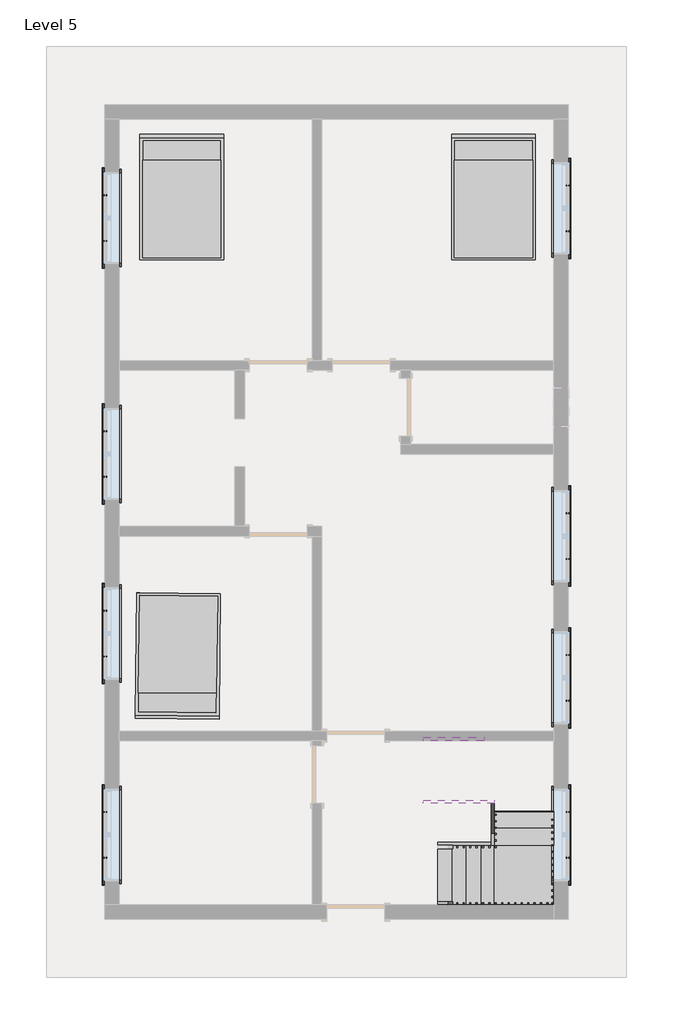
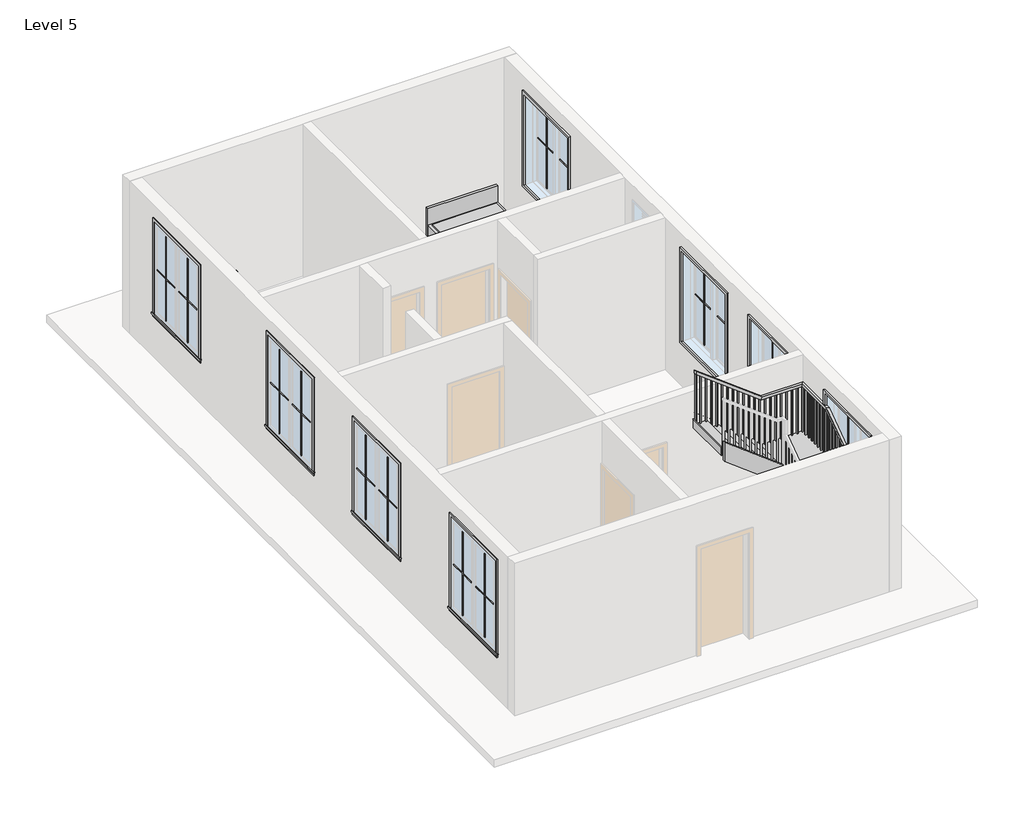
# One storey, part 2 of 2: 32 proxies, 5 members, 3 furniture elements, 1 railing, 1 stair flight.
"""IFC4 building model written with IfcOpenShell, lengths in millimetres."""

from ifc_helpers import new_model, si_unit, frame, origin, place, context, project, spatial, polyline, outline, extrude, faceted_brep, transform, mapped, element, save
from components import muntin_pattern_2x2_muntin_pattern_2x2_bff912c5, muntin_pattern_2x2_muntin_pattern_2x2_c2194282, trim_window_exterior_flat_with_sill_e04b3088, trim_window_interior_flat_picture_frame_2a7685fe, bed_17739_bed_17739_15c61121, stair_flight_f19c2654

model = new_model("IFC4")

# Units and contexts
model_context = context("Model", 3, world=origin())
ifc_project = project(units=[si_unit("LENGTHUNIT", "METRE", prefix="MILLI")], contexts=[model_context])

# Site, building, storey
site = spatial("IfcSite", under=ifc_project)
building = spatial("IfcBuilding", under=site)
storey = spatial("IfcBuildingStorey", under=building, Name="Level 5", Elevation=9601.2)

# Proxies
placement = place(None, origin())
muntin_pattern_2x2_muntin_pattern_2x2_shape = muntin_pattern_2x2_muntin_pattern_2x2_bff912c5(model_context)
element("IfcBuildingElementProxy", 1, Name="Muntin Pattern_2x2 : Muntin Pattern_2x2", ObjectType="Muntin Pattern_2x2 : Muntin Pattern_2x2", at=placement, inside=storey, context=model_context, shape_type="MappedRepresentation", body=[
    mapped(muntin_pattern_2x2_muntin_pattern_2x2_shape, transform((-4903.510885, -5396.5975571, 10585.45), x_axis=(0.0, 1.0, 0.0), y_axis=(-1.0, 0.0, 0.0), z_axis=(0.0, 0.0, 1.0))),
])
element("IfcBuildingElementProxy", 2, Name="Muntin Pattern_2x2 : Muntin Pattern_2x2", ObjectType="Muntin Pattern_2x2 : Muntin Pattern_2x2", at=placement, inside=storey, context=model_context, shape_type="MappedRepresentation", body=[
    mapped(muntin_pattern_2x2_muntin_pattern_2x2_shape, transform((2392.639115, -4675.8725571, 10585.45), x_axis=(0.0, -1.0, 0.0), y_axis=(1.0, 0.0, 0.0), z_axis=(0.0, 0.0, 1.0))),
])
element("IfcBuildingElementProxy", 3, Name="Muntin Pattern_2x2 : Muntin Pattern_2x2", ObjectType="Muntin Pattern_2x2 : Muntin Pattern_2x2", at=placement, inside=storey, context=model_context, shape_type="MappedRepresentation", body=[
    mapped(muntin_pattern_2x2_muntin_pattern_2x2_shape, transform((2392.639115, -2199.3725571, 10585.45), x_axis=(0.0, -1.0, 0.0), y_axis=(1.0, 0.0, 0.0), z_axis=(0.0, 0.0, 1.0))),
])
element("IfcBuildingElementProxy", 4, Name="Muntin Pattern_2x2 : Muntin Pattern_2x2", ObjectType="Muntin Pattern_2x2 : Muntin Pattern_2x2", at=placement, inside=storey, context=model_context, shape_type="MappedRepresentation", body=[
    mapped(muntin_pattern_2x2_muntin_pattern_2x2_shape, transform((2392.639115, 35.8274429, 10585.45), x_axis=(0.0, -1.0, 0.0), y_axis=(1.0, 0.0, 0.0), z_axis=(0.0, 0.0, 1.0))),
])
element("IfcBuildingElementProxy", 5, Name="Muntin Pattern_2x2 : Muntin Pattern_2x2", ObjectType="Muntin Pattern_2x2 : Muntin Pattern_2x2", at=placement, inside=storey, context=model_context, shape_type="MappedRepresentation", body=[
    mapped(muntin_pattern_2x2_muntin_pattern_2x2_shape, transform((-4903.510885, -2221.5975571, 10585.45), x_axis=(0.0, 1.0, 0.0), y_axis=(-1.0, 0.0, 0.0), z_axis=(0.0, 0.0, 1.0))),
])
element("IfcBuildingElementProxy", 6, Name="Muntin Pattern_2x2 : Muntin Pattern_2x2", ObjectType="Muntin Pattern_2x2 : Muntin Pattern_2x2", at=placement, inside=storey, context=model_context, shape_type="MappedRepresentation", body=[
    mapped(muntin_pattern_2x2_muntin_pattern_2x2_shape, transform((-4903.510885, 610.5024429, 10585.45), x_axis=(0.0, 1.0, 0.0), y_axis=(-1.0, 0.0, 0.0), z_axis=(0.0, 0.0, 1.0))),
])
element("IfcBuildingElementProxy", 7, Name="Muntin Pattern_2x2 : Muntin Pattern_2x2", ObjectType="Muntin Pattern_2x2 : Muntin Pattern_2x2", at=placement, inside=storey, context=model_context, shape_type="MappedRepresentation", body=[
    mapped(muntin_pattern_2x2_muntin_pattern_2x2_shape, transform((-4903.510885, 4331.6024429, 10585.45), x_axis=(0.0, 1.0, 0.0), y_axis=(-1.0, 0.0, 0.0), z_axis=(0.0, 0.0, 1.0))),
])
element("IfcBuildingElementProxy", 8, Name="Muntin Pattern_2x2 : Muntin Pattern_2x2", ObjectType="Muntin Pattern_2x2 : Muntin Pattern_2x2", at=placement, inside=storey, context=model_context, shape_type="MappedRepresentation", body=[
    mapped(muntin_pattern_2x2_muntin_pattern_2x2_shape, transform((2392.639115, 5204.7274429, 10585.45), x_axis=(0.0, -1.0, 0.0), y_axis=(1.0, 0.0, 0.0), z_axis=(0.0, 0.0, 1.0))),
])
muntin_pattern_2x2_muntin_pattern_2x2_2_shape = muntin_pattern_2x2_muntin_pattern_2x2_c2194282(model_context)
element("IfcBuildingElementProxy", 9, Name="Muntin Pattern_2x2 : Muntin Pattern_2x2", ObjectType="Muntin Pattern_2x2 : Muntin Pattern_2x2", at=placement, inside=storey, context=model_context, shape_type="MappedRepresentation", body=[
    mapped(muntin_pattern_2x2_muntin_pattern_2x2_2_shape, transform((-4903.510885, -4675.8725571, 10585.45), x_axis=(0.0, -1.0, 0.0), y_axis=(1.0, 0.0, 0.0), z_axis=(0.0, 0.0, 1.0))),
])
element("IfcBuildingElementProxy", 10, Name="Muntin Pattern_2x2 : Muntin Pattern_2x2", ObjectType="Muntin Pattern_2x2 : Muntin Pattern_2x2", at=placement, inside=storey, context=model_context, shape_type="MappedRepresentation", body=[
    mapped(muntin_pattern_2x2_muntin_pattern_2x2_2_shape, transform((2392.639115, -5396.5975571, 10585.45), x_axis=(0.0, 1.0, 0.0), y_axis=(-1.0, 0.0, 0.0), z_axis=(0.0, 0.0, 1.0))),
])
element("IfcBuildingElementProxy", 11, Name="Muntin Pattern_2x2 : Muntin Pattern_2x2", ObjectType="Muntin Pattern_2x2 : Muntin Pattern_2x2", at=placement, inside=storey, context=model_context, shape_type="MappedRepresentation", body=[
    mapped(muntin_pattern_2x2_muntin_pattern_2x2_2_shape, transform((2392.639115, -2920.0975571, 10585.45), x_axis=(0.0, 1.0, 0.0), y_axis=(-1.0, 0.0, 0.0), z_axis=(0.0, 0.0, 1.0))),
])
element("IfcBuildingElementProxy", 12, Name="Muntin Pattern_2x2 : Muntin Pattern_2x2", ObjectType="Muntin Pattern_2x2 : Muntin Pattern_2x2", at=placement, inside=storey, context=model_context, shape_type="MappedRepresentation", body=[
    mapped(muntin_pattern_2x2_muntin_pattern_2x2_2_shape, transform((2392.639115, -684.8975571, 10585.45), x_axis=(0.0, 1.0, 0.0), y_axis=(-1.0, 0.0, 0.0), z_axis=(0.0, 0.0, 1.0))),
])
element("IfcBuildingElementProxy", 13, Name="Muntin Pattern_2x2 : Muntin Pattern_2x2", ObjectType="Muntin Pattern_2x2 : Muntin Pattern_2x2", at=placement, inside=storey, context=model_context, shape_type="MappedRepresentation", body=[
    mapped(muntin_pattern_2x2_muntin_pattern_2x2_2_shape, transform((-4903.510885, -1500.8725571, 10585.45), x_axis=(0.0, -1.0, 0.0), y_axis=(1.0, 0.0, 0.0), z_axis=(0.0, 0.0, 1.0))),
])
element("IfcBuildingElementProxy", 14, Name="Muntin Pattern_2x2 : Muntin Pattern_2x2", ObjectType="Muntin Pattern_2x2 : Muntin Pattern_2x2", at=placement, inside=storey, context=model_context, shape_type="MappedRepresentation", body=[
    mapped(muntin_pattern_2x2_muntin_pattern_2x2_2_shape, transform((-4903.510885, 1331.2274429, 10585.45), x_axis=(0.0, -1.0, 0.0), y_axis=(1.0, 0.0, 0.0), z_axis=(0.0, 0.0, 1.0))),
])
element("IfcBuildingElementProxy", 15, Name="Muntin Pattern_2x2 : Muntin Pattern_2x2", ObjectType="Muntin Pattern_2x2 : Muntin Pattern_2x2", at=placement, inside=storey, context=model_context, shape_type="MappedRepresentation", body=[
    mapped(muntin_pattern_2x2_muntin_pattern_2x2_2_shape, transform((-4903.510885, 5052.3274429, 10585.45), x_axis=(0.0, -1.0, 0.0), y_axis=(1.0, 0.0, 0.0), z_axis=(0.0, 0.0, 1.0))),
])
element("IfcBuildingElementProxy", 16, Name="Muntin Pattern_2x2 : Muntin Pattern_2x2", ObjectType="Muntin Pattern_2x2 : Muntin Pattern_2x2", at=placement, inside=storey, context=model_context, shape_type="MappedRepresentation", body=[
    mapped(muntin_pattern_2x2_muntin_pattern_2x2_2_shape, transform((2392.639115, 4484.0024429, 10585.45), x_axis=(0.0, 1.0, 0.0), y_axis=(-1.0, 0.0, 0.0), z_axis=(0.0, 0.0, 1.0))),
])
trim_window_exterior_flat_with_sill_shape = trim_window_exterior_flat_with_sill_e04b3088(model_context)
element("IfcBuildingElementProxy", 17, Name="Trim-Window-Exterior-Flat : with Sill", ObjectType="Trim-Window-Exterior-Flat : with Sill", at=placement, inside=storey, context=model_context, shape_type="MappedRepresentation", body=[
    mapped(trim_window_exterior_flat_with_sill_shape, transform((-4913.035885, -5036.2350571, 12344.4), x_axis=(0.0, -1.0, 0.0), y_axis=(0.0, 0.0, 1.0), z_axis=(-1.0, 0.0, 0.0))),
])
element("IfcBuildingElementProxy", 18, Name="Trim-Window-Exterior-Flat : with Sill", ObjectType="Trim-Window-Exterior-Flat : with Sill", at=placement, inside=storey, context=model_context, shape_type="MappedRepresentation", body=[
    mapped(trim_window_exterior_flat_with_sill_shape, transform((2402.164115, -5036.2350571, 12344.4), x_axis=(0.0, 1.0, 0.0), y_axis=(0.0, 0.0, 1.0), z_axis=(1.0, 0.0, 0.0))),
])
element("IfcBuildingElementProxy", 19, Name="Trim-Window-Exterior-Flat : with Sill", ObjectType="Trim-Window-Exterior-Flat : with Sill", at=placement, inside=storey, context=model_context, shape_type="MappedRepresentation", body=[
    mapped(trim_window_exterior_flat_with_sill_shape, transform((2402.164115, -2559.7350571, 12344.4), x_axis=(0.0, 1.0, 0.0), y_axis=(0.0, 0.0, 1.0), z_axis=(1.0, 0.0, 0.0))),
])
element("IfcBuildingElementProxy", 20, Name="Trim-Window-Exterior-Flat : with Sill", ObjectType="Trim-Window-Exterior-Flat : with Sill", at=placement, inside=storey, context=model_context, shape_type="MappedRepresentation", body=[
    mapped(trim_window_exterior_flat_with_sill_shape, transform((2402.164115, -324.5350571, 12344.4), x_axis=(0.0, 1.0, 0.0), y_axis=(0.0, 0.0, 1.0), z_axis=(1.0, 0.0, 0.0))),
])
element("IfcBuildingElementProxy", 21, Name="Trim-Window-Exterior-Flat : with Sill", ObjectType="Trim-Window-Exterior-Flat : with Sill", at=placement, inside=storey, context=model_context, shape_type="MappedRepresentation", body=[
    mapped(trim_window_exterior_flat_with_sill_shape, transform((-4913.035885, -1861.2350571, 12344.4), x_axis=(0.0, -1.0, 0.0), y_axis=(0.0, 0.0, 1.0), z_axis=(-1.0, 0.0, 0.0))),
])
element("IfcBuildingElementProxy", 22, Name="Trim-Window-Exterior-Flat : with Sill", ObjectType="Trim-Window-Exterior-Flat : with Sill", at=placement, inside=storey, context=model_context, shape_type="MappedRepresentation", body=[
    mapped(trim_window_exterior_flat_with_sill_shape, transform((-4913.035885, 970.8649429, 12344.4), x_axis=(0.0, -1.0, 0.0), y_axis=(0.0, 0.0, 1.0), z_axis=(-1.0, 0.0, 0.0))),
])
element("IfcBuildingElementProxy", 23, Name="Trim-Window-Exterior-Flat : with Sill", ObjectType="Trim-Window-Exterior-Flat : with Sill", at=placement, inside=storey, context=model_context, shape_type="MappedRepresentation", body=[
    mapped(trim_window_exterior_flat_with_sill_shape, transform((-4913.035885, 4691.9649429, 12344.4), x_axis=(0.0, -1.0, 0.0), y_axis=(0.0, 0.0, 1.0), z_axis=(-1.0, 0.0, 0.0))),
])
element("IfcBuildingElementProxy", 24, Name="Trim-Window-Exterior-Flat : with Sill", ObjectType="Trim-Window-Exterior-Flat : with Sill", at=placement, inside=storey, context=model_context, shape_type="MappedRepresentation", body=[
    mapped(trim_window_exterior_flat_with_sill_shape, transform((2402.164115, 4844.3649429, 12344.4), x_axis=(0.0, 1.0, 0.0), y_axis=(0.0, 0.0, 1.0), z_axis=(1.0, 0.0, 0.0))),
])
trim_window_interior_flat_picture_frame_shape = trim_window_interior_flat_picture_frame_2a7685fe(model_context)
element("IfcBuildingElementProxy", 25, Name="Trim-Window-Interior-Flat : Picture Frame", ObjectType="Trim-Window-Interior-Flat : Picture Frame", at=placement, inside=storey, context=model_context, shape_type="MappedRepresentation", body=[
    mapped(trim_window_interior_flat_picture_frame_shape, transform((-4684.435885, -5036.2350571, 12344.4), x_axis=(0.0, 1.0, 0.0), y_axis=(0.0, 0.0, 1.0), z_axis=(1.0, 0.0, 0.0))),
])
element("IfcBuildingElementProxy", 26, Name="Trim-Window-Interior-Flat : Picture Frame", ObjectType="Trim-Window-Interior-Flat : Picture Frame", at=placement, inside=storey, context=model_context, shape_type="MappedRepresentation", body=[
    mapped(trim_window_interior_flat_picture_frame_shape, transform((2173.564115, -5036.2350571, 12344.4), x_axis=(0.0, -1.0, 0.0), y_axis=(0.0, 0.0, 1.0), z_axis=(-1.0, 0.0, 0.0))),
])
element("IfcBuildingElementProxy", 27, Name="Trim-Window-Interior-Flat : Picture Frame", ObjectType="Trim-Window-Interior-Flat : Picture Frame", at=placement, inside=storey, context=model_context, shape_type="MappedRepresentation", body=[
    mapped(trim_window_interior_flat_picture_frame_shape, transform((2173.564115, -2559.7350571, 12344.4), x_axis=(0.0, -1.0, 0.0), y_axis=(0.0, 0.0, 1.0), z_axis=(-1.0, 0.0, 0.0))),
])
element("IfcBuildingElementProxy", 28, Name="Trim-Window-Interior-Flat : Picture Frame", ObjectType="Trim-Window-Interior-Flat : Picture Frame", at=placement, inside=storey, context=model_context, shape_type="MappedRepresentation", body=[
    mapped(trim_window_interior_flat_picture_frame_shape, transform((2173.564115, -324.5350571, 12344.4), x_axis=(0.0, -1.0, 0.0), y_axis=(0.0, 0.0, 1.0), z_axis=(-1.0, 0.0, 0.0))),
])
element("IfcBuildingElementProxy", 29, Name="Trim-Window-Interior-Flat : Picture Frame", ObjectType="Trim-Window-Interior-Flat : Picture Frame", at=placement, inside=storey, context=model_context, shape_type="MappedRepresentation", body=[
    mapped(trim_window_interior_flat_picture_frame_shape, transform((-4684.435885, -1861.2350571, 12344.4), x_axis=(0.0, 1.0, 0.0), y_axis=(0.0, 0.0, 1.0), z_axis=(1.0, 0.0, 0.0))),
])
element("IfcBuildingElementProxy", 30, Name="Trim-Window-Interior-Flat : Picture Frame", ObjectType="Trim-Window-Interior-Flat : Picture Frame", at=placement, inside=storey, context=model_context, shape_type="MappedRepresentation", body=[
    mapped(trim_window_interior_flat_picture_frame_shape, transform((-4684.435885, 970.8649429, 12344.4), x_axis=(0.0, 1.0, 0.0), y_axis=(0.0, 0.0, 1.0), z_axis=(1.0, 0.0, 0.0))),
])
element("IfcBuildingElementProxy", 31, Name="Trim-Window-Interior-Flat : Picture Frame", ObjectType="Trim-Window-Interior-Flat : Picture Frame", at=placement, inside=storey, context=model_context, shape_type="MappedRepresentation", body=[
    mapped(trim_window_interior_flat_picture_frame_shape, transform((-4684.435885, 4691.9649429, 12344.4), x_axis=(0.0, 1.0, 0.0), y_axis=(0.0, 0.0, 1.0), z_axis=(1.0, 0.0, 0.0))),
])
element("IfcBuildingElementProxy", 32, Name="Trim-Window-Interior-Flat : Picture Frame", ObjectType="Trim-Window-Interior-Flat : Picture Frame", at=placement, inside=storey, context=model_context, shape_type="MappedRepresentation", body=[
    mapped(trim_window_interior_flat_picture_frame_shape, transform((2173.564115, 4844.3649429, 12344.4), x_axis=(0.0, -1.0, 0.0), y_axis=(0.0, 0.0, 1.0), z_axis=(-1.0, 0.0, 0.0))),
])

# Furniture
bed_17739_bed_17739_shape = bed_17739_bed_17739_15c61121(model_context)
element("IfcFurniture", 33, ObjectType="Bed_17739 : Bed_17739", at=placement, inside=storey, context=model_context, shape_type="MappedRepresentation", body=[
    mapped(bed_17739_bed_17739_shape, transform((-3693.835885, 4996.7649429, 9601.2), x_axis=(1.0, 0.0, 0.0), y_axis=(0.0, 1.0, 0.0), z_axis=(0.0, 0.0, 1.0))),
])
element("IfcFurniture", 34, ObjectType="Bed_17739 : Bed_17739", at=placement, inside=storey, context=model_context, shape_type="MappedRepresentation", body=[
    mapped(bed_17739_bed_17739_shape, transform((1221.064115, 4996.7649429, 9601.2), x_axis=(1.0, 0.0, 0.0), y_axis=(0.0, 1.0, 0.0), z_axis=(0.0, 0.0, 1.0))),
])
element("IfcFurniture", 35, ObjectType="Bed_17739 : Bed_17739", at=placement, inside=storey, context=model_context, shape_type="MappedRepresentation", body=[
    mapped(bed_17739_bed_17739_shape, transform((-3756.0321663, -2189.364606, 9601.2), x_axis=(-0.9999334593473937, 0.011535895177843815, 0.0), y_axis=(-0.011535895177843815, -0.9999334593473937, 0.0), z_axis=(0.0, 0.0, 1.0))),
])

# Members
element("IfcMember", 36, ObjectType="Stringer - 2\" Width", at=placement, inside=storey, context=model_context, shape_type="SweptSolid", body=[
    extrude(outline(polyline([(9823.8959685, 344.764115), (9601.2, 344.764115), (9601.2, 555.1685253), (10084.1196844, 1182.964115), (10468.6651993, 1182.964115), (9823.8959685, 344.764115)])), frame((0.0, -5201.3350571, 0.0), z_axis=(0.0, 1.0, 0.0), x_axis=(0.0, 0.0, 1.0)), (0.0, 0.0, 1.0), 50.8),
])
element("IfcMember", 37, ObjectType="Stringer - 2\" Width", at=placement, inside=storey, context=model_context, shape_type="SweptSolid", body=[
    extrude(outline(polyline([(-5201.3350571, 10296.352716), (-5201.3350571, 10670.9225362), (-4540.9350571, 11142.6368219), (-4540.9350571, 10768.0670017), (-5201.3350571, 10296.352716)])), frame((1182.964115, 0.0, 0.0), z_axis=(1.0, 0.0, 0.0), x_axis=(0.0, 1.0, 0.0)), (0.0, 0.0, 1.0), 50.8),
])
element("IfcMember", 38, ObjectType="Stringer - 2\" Width", at=placement, inside=storey, context=model_context, shape_type="SweptSolid", body=[
    extrude(outline(polyline([(10970.3786616, 1233.764115), (11353.5668, 1233.764115), (12205.0715619, 116.164115), (11821.8834236, 116.164115), (10970.3786616, 1233.764115)])), frame((0.0, -4540.9350571, 0.0), z_axis=(0.0, 1.0, 0.0), x_axis=(0.0, 0.0, 1.0)), (0.0, 0.0, 1.0), 50.8),
])
element("IfcMember", 39, ObjectType="Stringer - 2\" Width", at=placement, inside=storey, context=model_context, shape_type="SweptSolid", body=[
    extrude(outline(polyline([(9823.8959685, 344.764115), (9601.2, 344.764115), (9601.2, 555.1685253), (9999.6368219, 1073.1363938), (9999.6368219, 573.2272245), (9823.8959685, 344.764115)])), frame((0.0, -6191.9350571, 0.0), z_axis=(0.0, 1.0, 0.0), x_axis=(0.0, 0.0, 1.0)), (0.0, 0.0, 1.0), 50.8),
])
element("IfcMember", 40, ObjectType="Stringer - 2\" Width", at=placement, inside=storey, context=model_context, shape_type="SweptSolid", body=[
    extrude(outline(polyline([(11475.6384303, 1073.5451003), (12205.0715619, 116.164115), (11821.8834236, 116.164115), (11475.6384303, 570.6106687), (11475.6384303, 1073.5451003)])), frame((0.0, -3550.3350571, 0.0), z_axis=(0.0, 1.0, 0.0), x_axis=(0.0, 0.0, 1.0)), (0.0, 0.0, 1.0), 50.8),
])

# Railing
element("IfcRailing", 41, ObjectType="Handrail - Rectangular", at=placement, inside=storey, context=model_context, shape_type="SolidModel", body=[
    faceted_brep([(344.764115, -6090.3350571, 10684.9333333), (344.764115, -6090.3350571, 10621.0686436), (344.764115, -6141.1350571, 10621.0686436), (344.764115, -6141.1350571, 10684.9333333), (1373.464115, -6090.3350571, 11468.7047619), (1390.6115203, -6090.3350571, 11417.9047619), (1390.6115203, -6141.1350571, 11417.9047619), (1373.464115, -6141.1350571, 11468.7047619), (2122.764115, -6090.3350571, 11468.7047619), (2122.764115, -6090.3350571, 11417.9047619), (2173.564115, -6141.1350571, 11417.9047619), (2173.564115, -6141.1350571, 11468.7047619), (2122.764115, -5289.3883904, 11468.7047619), (2122.764115, -5273.1087657, 11417.9047619), (2173.564115, -5273.1087657, 11417.9047619), (2173.564115, -5289.3883904, 11468.7047619), (2122.764115, -4399.3108146, 12104.4744589), (2122.764115, -4383.0311899, 12053.6744589), (2173.564115, -4383.0311899, 12053.6744589), (2173.564115, -4399.3108146, 12104.4744589), (2122.764115, -3601.1350571, 12104.4744589), (2122.764115, -3601.1350571, 12053.6744589), (2173.564115, -3550.3350571, 12053.6744589), (2173.564115, -3550.3350571, 12104.4744589), (1371.6498293, -3601.1350571, 12104.4744589), (1354.5800477, -3601.1350571, 12053.6744589), (1354.5800477, -3550.3350571, 12053.6744589), (1371.6498293, -3550.3350571, 12104.4744589), (116.164115, -3601.1350571, 13055.6), (116.164115, -3550.3350571, 13055.6), (116.164115, -3550.3350571, 12991.8683472), (116.164115, -3601.1350571, 12991.8683472)], [[[0, 1, 2, 3]], [[1, 0, 4, 5]], [[2, 1, 5, 6]], [[3, 2, 6, 7]], [[0, 3, 7, 4]], [[5, 4, 8, 9]], [[6, 5, 9, 10]], [[7, 6, 10, 11]], [[4, 7, 11, 8]], [[9, 8, 12, 13]], [[10, 9, 13, 14]], [[11, 10, 14, 15]], [[8, 11, 15, 12]], [[13, 12, 16, 17]], [[14, 13, 17, 18]], [[15, 14, 18, 19]], [[12, 15, 19, 16]], [[17, 16, 20, 21]], [[18, 17, 21, 22]], [[19, 18, 22, 23]], [[16, 19, 23, 20]], [[21, 20, 24, 25]], [[22, 21, 25, 26]], [[23, 22, 26, 27]], [[20, 23, 27, 24]], [[28, 29, 30, 31]], [[25, 24, 28, 31]], [[26, 25, 31, 30]], [[27, 26, 30, 29]], [[24, 27, 29, 28]]]),
    extrude(outline(polyline([(12907.6827412, 227.289115), (12922.1145594, 208.239115), (11971.8666667, 208.239115), (11971.8666667, 227.289115), (12907.6827412, 227.289115)])), frame((0.0, -3585.2600571, 0.0), z_axis=(0.0, 1.0, 0.0), x_axis=(0.0, 0.0, 1.0)), (0.0, 0.0, 1.0), 19.05),
    extrude(outline(polyline([(12830.7130442, 328.889115), (12845.1448624, 309.839115), (11971.8666667, 309.839115), (11971.8666667, 328.889115), (12830.7130442, 328.889115)])), frame((0.0, -3585.2600571, 0.0), z_axis=(0.0, 1.0, 0.0), x_axis=(0.0, 0.0, 1.0)), (0.0, 0.0, 1.0), 19.05),
    extrude(outline(polyline([(12753.7433472, 430.489115), (12768.1751654, 411.439115), (11802.5333333, 411.439115), (11802.5333333, 430.489115), (12753.7433472, 430.489115)])), frame((0.0, -3585.2600571, 0.0), z_axis=(0.0, 1.0, 0.0), x_axis=(0.0, 0.0, 1.0)), (0.0, 0.0, 1.0), 19.05),
    extrude(outline(polyline([(12676.7736503, 532.089115), (12691.2054685, 513.039115), (11802.5333333, 513.039115), (11802.5333333, 532.089115), (12676.7736503, 532.089115)])), frame((0.0, -3585.2600571, 0.0), z_axis=(0.0, 1.0, 0.0), x_axis=(0.0, 0.0, 1.0)), (0.0, 0.0, 1.0), 19.05),
    extrude(outline(polyline([(12599.8039533, 633.689115), (12614.2357715, 614.639115), (11633.2, 614.639115), (11633.2, 633.689115), (12599.8039533, 633.689115)])), frame((0.0, -3585.2600571, 0.0), z_axis=(0.0, 1.0, 0.0), x_axis=(0.0, 0.0, 1.0)), (0.0, 0.0, 1.0), 19.05),
    extrude(outline(polyline([(12522.8342563, 735.289115), (12537.2660745, 716.239115), (11633.2, 716.239115), (11633.2, 735.289115), (12522.8342563, 735.289115)])), frame((0.0, -3585.2600571, 0.0), z_axis=(0.0, 1.0, 0.0), x_axis=(0.0, 0.0, 1.0)), (0.0, 0.0, 1.0), 19.05),
    extrude(outline(polyline([(12445.8645594, 836.889115), (12460.2963775, 817.839115), (11463.8666667, 817.839115), (11463.8666667, 836.889115), (12445.8645594, 836.889115)])), frame((0.0, -3585.2600571, 0.0), z_axis=(0.0, 1.0, 0.0), x_axis=(0.0, 0.0, 1.0)), (0.0, 0.0, 1.0), 19.05),
    extrude(outline(polyline([(12368.8948624, 938.489115), (12383.3266806, 919.439115), (11463.8666667, 919.439115), (11463.8666667, 938.489115), (12368.8948624, 938.489115)])), frame((0.0, -3585.2600571, 0.0), z_axis=(0.0, 1.0, 0.0), x_axis=(0.0, 0.0, 1.0)), (0.0, 0.0, 1.0), 19.05),
    extrude(outline(polyline([(12291.9251654, 1040.089115), (12306.3569836, 1021.039115), (11463.8666667, 1021.039115), (11463.8666667, 1040.089115), (12291.9251654, 1040.089115)])), frame((0.0, -3585.2600571, 0.0), z_axis=(0.0, 1.0, 0.0), x_axis=(0.0, 0.0, 1.0)), (0.0, 0.0, 1.0), 19.05),
    extrude(outline(polyline([(12214.9554685, 1141.689115), (12229.3872866, 1122.639115), (11294.5333333, 1122.639115), (11294.5333333, 1141.689115), (12214.9554685, 1141.689115)])), frame((0.0, -3585.2600571, 0.0), z_axis=(0.0, 1.0, 0.0), x_axis=(0.0, 0.0, 1.0)), (0.0, 0.0, 1.0), 19.05),
    extrude(outline(polyline([(12137.9857715, 1243.289115), (12152.4175897, 1224.239115), (11294.5333333, 1224.239115), (11294.5333333, 1243.289115), (12137.9857715, 1243.289115)])), frame((0.0, -3585.2600571, 0.0), z_axis=(0.0, 1.0, 0.0), x_axis=(0.0, 0.0, 1.0)), (0.0, 0.0, 1.0), 19.05),
    extrude(outline(polyline([(12061.0160745, 1344.889115), (12075.4478927, 1325.839115), (11125.2, 1325.839115), (11125.2, 1344.889115), (12061.0160745, 1344.889115)])), frame((0.0, -3585.2600571, 0.0), z_axis=(0.0, 1.0, 0.0), x_axis=(0.0, 0.0, 1.0)), (0.0, 0.0, 1.0), 19.05),
    extrude(outline(polyline([(1446.489115, -3566.2100571), (1446.489115, -3585.2600571), (1427.439115, -3585.2600571), (1427.439115, -3566.2100571), (1446.489115, -3566.2100571)])), frame((0.0, 0.0, 11125.2), z_axis=(0.0, 0.0, 1.0), x_axis=(1.0, 0.0, 0.0)), (0.0, 0.0, 1.0), 928.4744589),
    extrude(outline(polyline([(1548.089115, -3566.2100571), (1548.089115, -3585.2600571), (1529.039115, -3585.2600571), (1529.039115, -3566.2100571), (1548.089115, -3566.2100571)])), frame((0.0, 0.0, 11125.2), z_axis=(0.0, 0.0, 1.0), x_axis=(1.0, 0.0, 0.0)), (0.0, 0.0, 1.0), 928.4744589),
    extrude(outline(polyline([(1649.689115, -3566.2100571), (1649.689115, -3585.2600571), (1630.639115, -3585.2600571), (1630.639115, -3566.2100571), (1649.689115, -3566.2100571)])), frame((0.0, 0.0, 11125.2), z_axis=(0.0, 0.0, 1.0), x_axis=(1.0, 0.0, 0.0)), (0.0, 0.0, 1.0), 928.4744589),
    extrude(outline(polyline([(1751.289115, -3566.2100571), (1751.289115, -3585.2600571), (1732.239115, -3585.2600571), (1732.239115, -3566.2100571), (1751.289115, -3566.2100571)])), frame((0.0, 0.0, 11125.2), z_axis=(0.0, 0.0, 1.0), x_axis=(1.0, 0.0, 0.0)), (0.0, 0.0, 1.0), 928.4744589),
    extrude(outline(polyline([(1852.889115, -3566.2100571), (1852.889115, -3585.2600571), (1833.839115, -3585.2600571), (1833.839115, -3566.2100571), (1852.889115, -3566.2100571)])), frame((0.0, 0.0, 11125.2), z_axis=(0.0, 0.0, 1.0), x_axis=(1.0, 0.0, 0.0)), (0.0, 0.0, 1.0), 928.4744589),
    extrude(outline(polyline([(1954.489115, -3566.2100571), (1954.489115, -3585.2600571), (1935.439115, -3585.2600571), (1935.439115, -3566.2100571), (1954.489115, -3566.2100571)])), frame((0.0, 0.0, 11125.2), z_axis=(0.0, 0.0, 1.0), x_axis=(1.0, 0.0, 0.0)), (0.0, 0.0, 1.0), 928.4744589),
    extrude(outline(polyline([(2056.089115, -3566.2100571), (2056.089115, -3585.2600571), (2037.039115, -3585.2600571), (2037.039115, -3566.2100571), (2056.089115, -3566.2100571)])), frame((0.0, 0.0, 11125.2), z_axis=(0.0, 0.0, 1.0), x_axis=(1.0, 0.0, 0.0)), (0.0, 0.0, 1.0), 928.4744589),
    extrude(outline(polyline([(2157.689115, -3686.8600571), (2138.639115, -3686.8600571), (2138.639115, -3667.8100571), (2157.689115, -3667.8100571), (2157.689115, -3686.8600571)])), frame((0.0, 0.0, 11125.2), z_axis=(0.0, 0.0, 1.0), x_axis=(1.0, 0.0, 0.0)), (0.0, 0.0, 1.0), 928.4744589),
    extrude(outline(polyline([(2157.689115, -3788.4600571), (2138.639115, -3788.4600571), (2138.639115, -3769.4100571), (2157.689115, -3769.4100571), (2157.689115, -3788.4600571)])), frame((0.0, 0.0, 11125.2), z_axis=(0.0, 0.0, 1.0), x_axis=(1.0, 0.0, 0.0)), (0.0, 0.0, 1.0), 928.4744589),
    extrude(outline(polyline([(2157.689115, -3890.0600571), (2138.639115, -3890.0600571), (2138.639115, -3871.0100571), (2157.689115, -3871.0100571), (2157.689115, -3890.0600571)])), frame((0.0, 0.0, 11125.2), z_axis=(0.0, 0.0, 1.0), x_axis=(1.0, 0.0, 0.0)), (0.0, 0.0, 1.0), 928.4744589),
    extrude(outline(polyline([(2157.689115, -3991.6600571), (2138.639115, -3991.6600571), (2138.639115, -3972.6100571), (2157.689115, -3972.6100571), (2157.689115, -3991.6600571)])), frame((0.0, 0.0, 11125.2), z_axis=(0.0, 0.0, 1.0), x_axis=(1.0, 0.0, 0.0)), (0.0, 0.0, 1.0), 928.4744589),
    extrude(outline(polyline([(2157.689115, -4093.2600571), (2138.639115, -4093.2600571), (2138.639115, -4074.2100571), (2157.689115, -4074.2100571), (2157.689115, -4093.2600571)])), frame((0.0, 0.0, 11125.2), z_axis=(0.0, 0.0, 1.0), x_axis=(1.0, 0.0, 0.0)), (0.0, 0.0, 1.0), 928.4744589),
    extrude(outline(polyline([(2157.689115, -4194.8600571), (2138.639115, -4194.8600571), (2138.639115, -4175.8100571), (2157.689115, -4175.8100571), (2157.689115, -4194.8600571)])), frame((0.0, 0.0, 11125.2), z_axis=(0.0, 0.0, 1.0), x_axis=(1.0, 0.0, 0.0)), (0.0, 0.0, 1.0), 928.4744589),
    extrude(outline(polyline([(2157.689115, -4296.4600571), (2138.639115, -4296.4600571), (2138.639115, -4277.4100571), (2157.689115, -4277.4100571), (2157.689115, -4296.4600571)])), frame((0.0, 0.0, 11125.2), z_axis=(0.0, 0.0, 1.0), x_axis=(1.0, 0.0, 0.0)), (0.0, 0.0, 1.0), 928.4744589),
    extrude(outline(polyline([(2157.689115, -4398.0600571), (2138.639115, -4398.0600571), (2138.639115, -4379.0100571), (2157.689115, -4379.0100571), (2157.689115, -4398.0600571)])), frame((0.0, 0.0, 11125.2), z_axis=(0.0, 0.0, 1.0), x_axis=(1.0, 0.0, 0.0)), (0.0, 0.0, 1.0), 928.4744589),
    extrude(outline(polyline([(-4499.6600571, 11970.3681252), (-4480.6100571, 11983.9752681), (-4480.6100571, 11125.2), (-4499.6600571, 11125.2), (-4499.6600571, 11970.3681252)])), frame((2138.639115, 0.0, 0.0), z_axis=(1.0, 0.0, 0.0), x_axis=(0.0, 1.0, 0.0)), (0.0, 0.0, 1.0), 19.05),
    extrude(outline(polyline([(-4601.2600571, 11897.7966966), (-4582.2100571, 11911.4038395), (-4582.2100571, 10955.8666667), (-4601.2600571, 10955.8666667), (-4601.2600571, 11897.7966966)])), frame((2138.639115, 0.0, 0.0), z_axis=(1.0, 0.0, 0.0), x_axis=(0.0, 1.0, 0.0)), (0.0, 0.0, 1.0), 19.05),
    extrude(outline(polyline([(-4702.8600571, 11825.2252681), (-4683.8100571, 11838.8324109), (-4683.8100571, 10955.8666667), (-4702.8600571, 10955.8666667), (-4702.8600571, 11825.2252681)])), frame((2138.639115, 0.0, 0.0), z_axis=(1.0, 0.0, 0.0), x_axis=(0.0, 1.0, 0.0)), (0.0, 0.0, 1.0), 19.05),
    extrude(outline(polyline([(-4804.4600571, 11752.6538395), (-4785.4100571, 11766.2609823), (-4785.4100571, 10786.5333333), (-4804.4600571, 10786.5333333), (-4804.4600571, 11752.6538395)])), frame((2138.639115, 0.0, 0.0), z_axis=(1.0, 0.0, 0.0), x_axis=(0.0, 1.0, 0.0)), (0.0, 0.0, 1.0), 19.05),
    extrude(outline(polyline([(-4906.0600571, 11680.0824109), (-4887.0100571, 11693.6895538), (-4887.0100571, 10786.5333333), (-4906.0600571, 10786.5333333), (-4906.0600571, 11680.0824109)])), frame((2138.639115, 0.0, 0.0), z_axis=(1.0, 0.0, 0.0), x_axis=(0.0, 1.0, 0.0)), (0.0, 0.0, 1.0), 19.05),
    extrude(outline(polyline([(-5007.6600571, 11607.5109823), (-4988.6100571, 11621.1181252), (-4988.6100571, 10617.2), (-5007.6600571, 10617.2), (-5007.6600571, 11607.5109823)])), frame((2138.639115, 0.0, 0.0), z_axis=(1.0, 0.0, 0.0), x_axis=(0.0, 1.0, 0.0)), (0.0, 0.0, 1.0), 19.05),
    extrude(outline(polyline([(-5109.2600571, 11534.9395538), (-5090.2100571, 11548.5466966), (-5090.2100571, 10617.2), (-5109.2600571, 10617.2), (-5109.2600571, 11534.9395538)])), frame((2138.639115, 0.0, 0.0), z_axis=(1.0, 0.0, 0.0), x_axis=(0.0, 1.0, 0.0)), (0.0, 0.0, 1.0), 19.05),
    extrude(outline(polyline([(-5210.8600571, 11462.3681252), (-5191.8100571, 11475.9752681), (-5191.8100571, 10617.2), (-5210.8600571, 10617.2), (-5210.8600571, 11462.3681252)])), frame((2138.639115, 0.0, 0.0), z_axis=(1.0, 0.0, 0.0), x_axis=(0.0, 1.0, 0.0)), (0.0, 0.0, 1.0), 19.05),
    extrude(outline(polyline([(2157.689115, -5312.4600571), (2138.639115, -5312.4600571), (2138.639115, -5293.4100571), (2157.689115, -5293.4100571), (2157.689115, -5312.4600571)])), frame((0.0, 0.0, 10447.8666667), z_axis=(0.0, 0.0, 1.0), x_axis=(1.0, 0.0, 0.0)), (0.0, 0.0, 1.0), 970.0380952),
    extrude(outline(polyline([(2157.689115, -5414.0600571), (2138.639115, -5414.0600571), (2138.639115, -5395.0100571), (2157.689115, -5395.0100571), (2157.689115, -5414.0600571)])), frame((0.0, 0.0, 10447.8666667), z_axis=(0.0, 0.0, 1.0), x_axis=(1.0, 0.0, 0.0)), (0.0, 0.0, 1.0), 970.0380952),
    extrude(outline(polyline([(2157.689115, -5515.6600571), (2138.639115, -5515.6600571), (2138.639115, -5496.6100571), (2157.689115, -5496.6100571), (2157.689115, -5515.6600571)])), frame((0.0, 0.0, 10447.8666667), z_axis=(0.0, 0.0, 1.0), x_axis=(1.0, 0.0, 0.0)), (0.0, 0.0, 1.0), 970.0380952),
    extrude(outline(polyline([(2157.689115, -5617.2600571), (2138.639115, -5617.2600571), (2138.639115, -5598.2100571), (2157.689115, -5598.2100571), (2157.689115, -5617.2600571)])), frame((0.0, 0.0, 10447.8666667), z_axis=(0.0, 0.0, 1.0), x_axis=(1.0, 0.0, 0.0)), (0.0, 0.0, 1.0), 970.0380952),
    extrude(outline(polyline([(2157.689115, -5718.8600571), (2138.639115, -5718.8600571), (2138.639115, -5699.8100571), (2157.689115, -5699.8100571), (2157.689115, -5718.8600571)])), frame((0.0, 0.0, 10447.8666667), z_axis=(0.0, 0.0, 1.0), x_axis=(1.0, 0.0, 0.0)), (0.0, 0.0, 1.0), 970.0380952),
    extrude(outline(polyline([(2157.689115, -5820.4600571), (2138.639115, -5820.4600571), (2138.639115, -5801.4100571), (2157.689115, -5801.4100571), (2157.689115, -5820.4600571)])), frame((0.0, 0.0, 10447.8666667), z_axis=(0.0, 0.0, 1.0), x_axis=(1.0, 0.0, 0.0)), (0.0, 0.0, 1.0), 970.0380952),
    extrude(outline(polyline([(2157.689115, -5922.0600571), (2138.639115, -5922.0600571), (2138.639115, -5903.0100571), (2157.689115, -5903.0100571), (2157.689115, -5922.0600571)])), frame((0.0, 0.0, 10447.8666667), z_axis=(0.0, 0.0, 1.0), x_axis=(1.0, 0.0, 0.0)), (0.0, 0.0, 1.0), 970.0380952),
    extrude(outline(polyline([(2157.689115, -6023.6600571), (2138.639115, -6023.6600571), (2138.639115, -6004.6100571), (2157.689115, -6004.6100571), (2157.689115, -6023.6600571)])), frame((0.0, 0.0, 10447.8666667), z_axis=(0.0, 0.0, 1.0), x_axis=(1.0, 0.0, 0.0)), (0.0, 0.0, 1.0), 970.0380952),
    extrude(outline(polyline([(2062.439115, -6125.2600571), (2062.439115, -6106.2100571), (2081.489115, -6106.2100571), (2081.489115, -6125.2600571), (2062.439115, -6125.2600571)])), frame((0.0, 0.0, 10447.8666667), z_axis=(0.0, 0.0, 1.0), x_axis=(1.0, 0.0, 0.0)), (0.0, 0.0, 1.0), 970.0380952),
    extrude(outline(polyline([(1960.839115, -6125.2600571), (1960.839115, -6106.2100571), (1979.889115, -6106.2100571), (1979.889115, -6125.2600571), (1960.839115, -6125.2600571)])), frame((0.0, 0.0, 10447.8666667), z_axis=(0.0, 0.0, 1.0), x_axis=(1.0, 0.0, 0.0)), (0.0, 0.0, 1.0), 970.0380952),
    extrude(outline(polyline([(1859.239115, -6125.2600571), (1859.239115, -6106.2100571), (1878.289115, -6106.2100571), (1878.289115, -6125.2600571), (1859.239115, -6125.2600571)])), frame((0.0, 0.0, 10447.8666667), z_axis=(0.0, 0.0, 1.0), x_axis=(1.0, 0.0, 0.0)), (0.0, 0.0, 1.0), 970.0380952),
    extrude(outline(polyline([(1757.639115, -6125.2600571), (1757.639115, -6106.2100571), (1776.689115, -6106.2100571), (1776.689115, -6125.2600571), (1757.639115, -6125.2600571)])), frame((0.0, 0.0, 10447.8666667), z_axis=(0.0, 0.0, 1.0), x_axis=(1.0, 0.0, 0.0)), (0.0, 0.0, 1.0), 970.0380952),
    extrude(outline(polyline([(1656.039115, -6125.2600571), (1656.039115, -6106.2100571), (1675.089115, -6106.2100571), (1675.089115, -6125.2600571), (1656.039115, -6125.2600571)])), frame((0.0, 0.0, 10447.8666667), z_axis=(0.0, 0.0, 1.0), x_axis=(1.0, 0.0, 0.0)), (0.0, 0.0, 1.0), 970.0380952),
    extrude(outline(polyline([(1554.439115, -6125.2600571), (1554.439115, -6106.2100571), (1573.489115, -6106.2100571), (1573.489115, -6125.2600571), (1554.439115, -6125.2600571)])), frame((0.0, 0.0, 10447.8666667), z_axis=(0.0, 0.0, 1.0), x_axis=(1.0, 0.0, 0.0)), (0.0, 0.0, 1.0), 970.0380952),
    extrude(outline(polyline([(1452.839115, -6125.2600571), (1452.839115, -6106.2100571), (1471.889115, -6106.2100571), (1471.889115, -6125.2600571), (1452.839115, -6125.2600571)])), frame((0.0, 0.0, 10447.8666667), z_axis=(0.0, 0.0, 1.0), x_axis=(1.0, 0.0, 0.0)), (0.0, 0.0, 1.0), 970.0380952),
    extrude(outline(polyline([(11402.4210246, 1370.289115), (11387.9067388, 1351.239115), (10447.8666667, 1351.239115), (10447.8666667, 1370.289115), (11402.4210246, 1370.289115)])), frame((0.0, -6125.2600571, 0.0), z_axis=(0.0, 1.0, 0.0), x_axis=(0.0, 0.0, 1.0)), (0.0, 0.0, 1.0), 19.05),
    extrude(outline(polyline([(11325.0115007, 1268.689115), (11310.497215, 1249.639115), (10447.8666667, 1249.639115), (10447.8666667, 1268.689115), (11325.0115007, 1268.689115)])), frame((0.0, -6125.2600571, 0.0), z_axis=(0.0, 1.0, 0.0), x_axis=(0.0, 0.0, 1.0)), (0.0, 0.0, 1.0), 19.05),
    extrude(outline(polyline([(11247.6019769, 1167.089115), (11233.0876912, 1148.039115), (10278.5333333, 1148.039115), (10278.5333333, 1167.089115), (11247.6019769, 1167.089115)])), frame((0.0, -6125.2600571, 0.0), z_axis=(0.0, 1.0, 0.0), x_axis=(0.0, 0.0, 1.0)), (0.0, 0.0, 1.0), 19.05),
    extrude(outline(polyline([(11170.1924531, 1065.489115), (11155.6781674, 1046.439115), (10278.5333333, 1046.439115), (10278.5333333, 1065.489115), (11170.1924531, 1065.489115)])), frame((0.0, -6125.2600571, 0.0), z_axis=(0.0, 1.0, 0.0), x_axis=(0.0, 0.0, 1.0)), (0.0, 0.0, 1.0), 19.05),
    extrude(outline(polyline([(11092.7829293, 963.889115), (11078.2686436, 944.839115), (10109.2, 944.839115), (10109.2, 963.889115), (11092.7829293, 963.889115)])), frame((0.0, -6125.2600571, 0.0), z_axis=(0.0, 1.0, 0.0), x_axis=(0.0, 0.0, 1.0)), (0.0, 0.0, 1.0), 19.05),
    extrude(outline(polyline([(11015.3734055, 862.289115), (11000.8591198, 843.239115), (10109.2, 843.239115), (10109.2, 862.289115), (11015.3734055, 862.289115)])), frame((0.0, -6125.2600571, 0.0), z_axis=(0.0, 1.0, 0.0), x_axis=(0.0, 0.0, 1.0)), (0.0, 0.0, 1.0), 19.05),
    extrude(outline(polyline([(10937.9638817, 760.689115), (10923.449596, 741.639115), (9939.8666667, 741.639115), (9939.8666667, 760.689115), (10937.9638817, 760.689115)])), frame((0.0, -6125.2600571, 0.0), z_axis=(0.0, 1.0, 0.0), x_axis=(0.0, 0.0, 1.0)), (0.0, 0.0, 1.0), 19.05),
    extrude(outline(polyline([(10860.5543579, 659.089115), (10846.0400722, 640.039115), (9939.8666667, 640.039115), (9939.8666667, 659.089115), (10860.5543579, 659.089115)])), frame((0.0, -6125.2600571, 0.0), z_axis=(0.0, 1.0, 0.0), x_axis=(0.0, 0.0, 1.0)), (0.0, 0.0, 1.0), 19.05),
    extrude(outline(polyline([(10783.1448341, 557.489115), (10768.6305484, 538.439115), (9770.5333333, 538.439115), (9770.5333333, 557.489115), (10783.1448341, 557.489115)])), frame((0.0, -6125.2600571, 0.0), z_axis=(0.0, 1.0, 0.0), x_axis=(0.0, 0.0, 1.0)), (0.0, 0.0, 1.0), 19.05),
    extrude(outline(polyline([(10705.7353103, 455.889115), (10691.2210246, 436.839115), (9770.5333333, 436.839115), (9770.5333333, 455.889115), (10705.7353103, 455.889115)])), frame((0.0, -6125.2600571, 0.0), z_axis=(0.0, 1.0, 0.0), x_axis=(0.0, 0.0, 1.0)), (0.0, 0.0, 1.0), 19.05),
    extrude(outline(polyline([(2157.689115, -3585.2600571), (2138.639115, -3585.2600571), (2138.639115, -3566.2100571), (2157.689115, -3566.2100571), (2157.689115, -3585.2600571)])), frame((0.0, 0.0, 11125.2), z_axis=(0.0, 0.0, 1.0), x_axis=(1.0, 0.0, 0.0)), (0.0, 0.0, 1.0), 928.4744589),
    extrude(outline(polyline([(2138.639115, -6125.2600571), (2138.639115, -6106.2100571), (2157.689115, -6106.2100571), (2157.689115, -6125.2600571), (2138.639115, -6125.2600571)])), frame((0.0, 0.0, 10447.8666667), z_axis=(0.0, 0.0, 1.0), x_axis=(1.0, 0.0, 0.0)), (0.0, 0.0, 1.0), 970.0380952),
    extrude(outline(polyline([(12977.4365291, 135.214115), (12991.8683472, 116.164115), (11971.8666667, 116.164115), (11971.8666667, 135.214115), (12977.4365291, 135.214115)])), frame((0.0, -3585.2600571, 0.0), z_axis=(0.0, 1.0, 0.0), x_axis=(0.0, 0.0, 1.0)), (0.0, 0.0, 1.0), 19.05),
    extrude(outline(polyline([(10635.5829293, 363.814115), (10621.0686436, 344.764115), (9770.5333333, 344.764115), (9770.5333333, 363.814115), (10635.5829293, 363.814115)])), frame((0.0, -6125.2600571, 0.0), z_axis=(0.0, 1.0, 0.0), x_axis=(0.0, 0.0, 1.0)), (0.0, 0.0, 1.0), 19.05),
])

# Stair flight
stair_flight_shape = stair_flight_f19c2654(model_context)
element("IfcStairFlight", 42, ObjectType="2\" Tread 1\" Nosing 1/4\" Riser", at=placement, inside=storey, context=model_context, shape_type="MappedRepresentation", body=[
    mapped(stair_flight_shape, transform((0.0, 0.0, 0.0), x_axis=(1.0, 0.0, 0.0), y_axis=(0.0, 1.0, 0.0), z_axis=(0.0, 0.0, 1.0))),
])

save(model, "model.ifc")

# Revit data of these elements
# Type "Muntin Pattern_2x2 : Muntin Pattern_2x2"
#   Width [instance default] = 4' - 0"
#   Thickness = 0' - 0 1/2"
#   Height [instance default] = 4' - 0"
#   Distance = 0' - 0 3/4"
#   Interior Material [instance default] = none
#   Exterior Material [instance default] = none
#   Default Elevation = 0
# Type "Trim-Window-Exterior-Flat : with Sill"
#   Trim Width = 0' - 2 1/4"
#   Trim Thickness_Picture Frame = 0' - 1 1/4"
#   Trim Thickness_with Sill = 0' - 0 3/4"
#   Sill Thickness = 0' - 1 1/4"
#   Opening Width [instance default] = 2' - 0"
#   Opening Height [instance default] = 3' - 0"
#   Default Elevation = 4' - 0"
#   Sill = yes
#   Picture Frame = no
#   Trim Material [instance default] = none
# Type "Trim-Window-Interior-Flat : Picture Frame"
#   Trim Thickness_Picture Frame = 0' - 1 1/4"
#   Trim Width = 0' - 2 1/4"
#   Trim Thickness_with Sill = 0' - 0 3/4"
#   Sill Thickness = 0' - 1 1/4"
#   Opening Width [instance default] = 2' - 0"
#   Opening Height [instance default] = 3' - 0"
#   Default Elevation = 4' - 0"
#   Sill = no
#   Picture Frame = yes
#   Trim Material [instance default] = none
# Type "Bed_17739 : Bed_17739"
#   Default Elevation = 0
# Type "Handrail - Rectangular"
#   Assembly Code = "C2010400"
#   built-in parameter 1008612 = 0.0416667 (stored number, unit not read)
#   built-in parameter 1008611 = 0.0416667 (stored number, unit not read)
#   built-in parameter 1008609 = 0.333333 (stored number, unit not read)
#   built-in parameter 1008604 = 0.166667 (stored number, unit not read)
#   built-in parameter 1008603 = 0.166667 (stored number, unit not read)
#   Railing Height = 3' - 0"
#   built-in parameter 1008630 = 2
#   built-in parameter 1008610 = 2
#   built-in parameter 1008618 = Baluster - Square : 3/4"
# Elements 1, 2, 3, 4, 5, 6, 7, 8, 9, 10, 11, 12, 13, 14, 15, 16 (IfcBuildingElementProxy, "Muntin Pattern_2x2 : Muntin Pattern_2x2")
#   Width = 1' - 11 1/8"
#   Height = 5' - 6 1/2"
#   Interior Material = Wood - Stained
#   Exterior Material = Clad - White
#   Phase Created = New Construction
#   Materials on its faces: "Clad - White", "Wood - Stained"
# Elements 17, 18, 19, 20, 21, 22, 23, 24 (IfcBuildingElementProxy, "Trim-Window-Exterior-Flat : with Sill")
#   Opening Width = 4' - 9"
#   Opening Height = 6' - 0"
#   Trim Material = Clad - White
#   Phase Created = New Construction
#   Materials on its faces: "Clad - White"
# Elements 25, 26, 27, 28, 29, 30, 31, 32 (IfcBuildingElementProxy, "Trim-Window-Interior-Flat : Picture Frame")
#   Opening Width = 4' - 9"
#   Opening Height = 6' - 0"
#   Trim Material = Wood - Stained
#   Phase Created = New Construction
#   Materials on its faces: "Wood - Stained"
# Elements 33, 34, 35 (IfcFurniture, "Bed_17739 : Bed_17739")
#   Phase Created = New Construction
#   Materials on its faces: "legs", "sheets", "bed frame", "Blanket"
# Elements 36, 37, 38, 39, 40 (IfcMember, "Stringer - 2\" Width")
#   Phase Created = New Construction
# Element 41 (IfcRailing, "Handrail - Rectangular")
#   Phase Created = New Construction
# Element 42 (IfcStairFlight, "2\" Tread 1\" Nosing 1/4\" Riser")
#   Phase Created = New Construction
# Materials
#   "Clad - White": class "Wood", colour RGB 242 242 238, transparency 0, Cost = 0
#   "Wood - Stained": class "Wood", colour RGB 224 178 126, transparency 0, Cost = 0
#   "legs": colour RGB 90 73 37, transparency 0, Cost = 0
#   "sheets": colour RGB 200 195 176, transparency 0, Cost = 0
#   "bed frame": colour RGB 90 73 37, transparency 0, Cost = 0
#   "Blanket": class "System", colour RGB 59 0 1, transparency 0, Cost = 0
